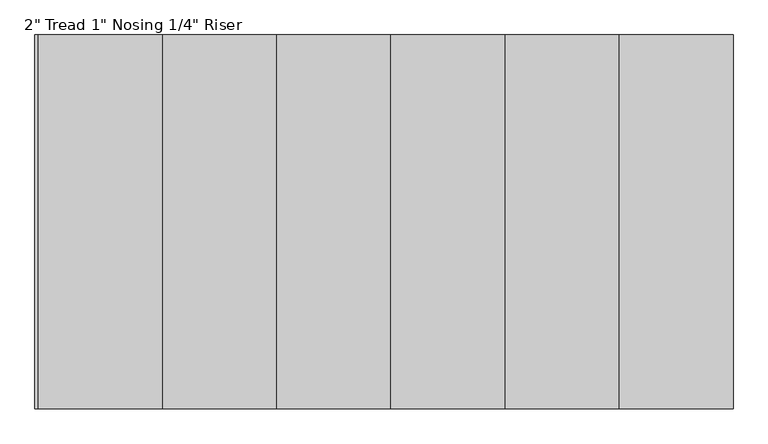
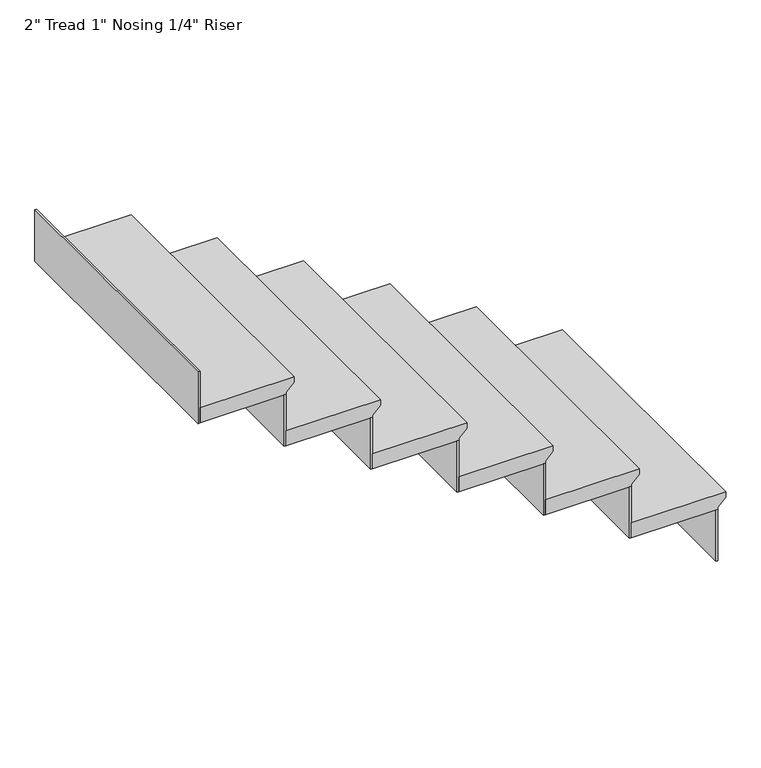
"""IFC4 building model written with IfcOpenShell, lengths in millimetres: stair flight geometry."""

from ifc_helpers import new_model, si_unit, frame, origin, place, context, project, spatial, polyline, outline, extrude, source, transform, mapped, element, save


def stair_flight_8de20f2d(model_context):
    return source(origin(), model_context, "Body", "SweptSolid", [
        extrude(outline(polyline([(5646.8210526, 8676.6463344), (5646.8210526, 8371.8463344), (5596.0210526, 8371.8463344), (5596.0210526, 8651.2463344), (5602.3710526, 8651.2463344), (5627.7710526, 8676.6463344), (5646.8210526, 8676.6463344)])), frame((0.0, -8089.9746824, 0.0), z_axis=(0.0, 1.0, 0.0), x_axis=(0.0, 0.0, 1.0)), (0.0, 0.0, 1.0), 914.4),
        extrude(outline(polyline([(8644.8963344, -7175.5746824), (8651.2463344, -7175.5746824), (8651.2463344, -8089.9746824), (8644.8963344, -8089.9746824), (8644.8963344, -7175.5746824)])), frame((0.0, 0.0, 5419.5578947), z_axis=(0.0, 0.0, 1.0), x_axis=(1.0, 0.0, 0.0)), (0.0, 0.0, 1.0), 176.4631579),
        extrude(outline(polyline([(8365.4963344, -7175.5746824), (8371.8463344, -7175.5746824), (8371.8463344, -8089.9746824), (8365.4963344, -8089.9746824), (8365.4963344, -7175.5746824)])), frame((0.0, 0.0, 5596.0210526), z_axis=(0.0, 0.0, 1.0), x_axis=(1.0, 0.0, 0.0)), (0.0, 0.0, 1.0), 176.4631579),
        extrude(outline(polyline([(5823.2842105, 8397.2463344), (5823.2842105, 8092.4463344), (5772.4842105, 8092.4463344), (5772.4842105, 8371.8463344), (5778.8342105, 8371.8463344), (5804.2342105, 8397.2463344), (5823.2842105, 8397.2463344)])), frame((0.0, -8089.9746824, 0.0), z_axis=(0.0, 1.0, 0.0), x_axis=(0.0, 0.0, 1.0)), (0.0, 0.0, 1.0), 914.4),
        extrude(outline(polyline([(8086.0963344, -7175.5746824), (8092.4463344, -7175.5746824), (8092.4463344, -8089.9746824), (8086.0963344, -8089.9746824), (8086.0963344, -7175.5746824)])), frame((0.0, 0.0, 5772.4842105), z_axis=(0.0, 0.0, 1.0), x_axis=(1.0, 0.0, 0.0)), (0.0, 0.0, 1.0), 176.4631579),
        extrude(outline(polyline([(5999.7473684, 8117.8463344), (5999.7473684, 7813.0463344), (5948.9473684, 7813.0463344), (5948.9473684, 8092.4463344), (5955.2973684, 8092.4463344), (5980.6973684, 8117.8463344), (5999.7473684, 8117.8463344)])), frame((0.0, -8089.9746824, 0.0), z_axis=(0.0, 1.0, 0.0), x_axis=(0.0, 0.0, 1.0)), (0.0, 0.0, 1.0), 914.4),
        extrude(outline(polyline([(7806.6963344, -7175.5746824), (7813.0463344, -7175.5746824), (7813.0463344, -8089.9746824), (7806.6963344, -8089.9746824), (7806.6963344, -7175.5746824)])), frame((0.0, 0.0, 5948.9473684), z_axis=(0.0, 0.0, 1.0), x_axis=(1.0, 0.0, 0.0)), (0.0, 0.0, 1.0), 176.4631579),
        extrude(outline(polyline([(6176.2105263, 7838.4463344), (6176.2105263, 7533.6463344), (6125.4105263, 7533.6463344), (6125.4105263, 7813.0463344), (6131.7605263, 7813.0463344), (6157.1605263, 7838.4463344), (6176.2105263, 7838.4463344)])), frame((0.0, -8089.9746824, 0.0), z_axis=(0.0, 1.0, 0.0), x_axis=(0.0, 0.0, 1.0)), (0.0, 0.0, 1.0), 914.4),
        extrude(outline(polyline([(7527.2963344, -7175.5746824), (7533.6463344, -7175.5746824), (7533.6463344, -8089.9746824), (7527.2963344, -8089.9746824), (7527.2963344, -7175.5746824)])), frame((0.0, 0.0, 6125.4105263), z_axis=(0.0, 0.0, 1.0), x_axis=(1.0, 0.0, 0.0)), (0.0, 0.0, 1.0), 176.4631579),
        extrude(outline(polyline([(6352.6736842, 7559.0463344), (6352.6736842, 7254.2463344), (6301.8736842, 7254.2463344), (6301.8736842, 7533.6463344), (6308.2236842, 7533.6463344), (6333.6236842, 7559.0463344), (6352.6736842, 7559.0463344)])), frame((0.0, -8089.9746824, 0.0), z_axis=(0.0, 1.0, 0.0), x_axis=(0.0, 0.0, 1.0)), (0.0, 0.0, 1.0), 914.4),
        extrude(outline(polyline([(7247.8963344, -7175.5746824), (7254.2463344, -7175.5746824), (7254.2463344, -8089.9746824), (7247.8963344, -8089.9746824), (7247.8963344, -7175.5746824)])), frame((0.0, 0.0, 6301.8736842), z_axis=(0.0, 0.0, 1.0), x_axis=(1.0, 0.0, 0.0)), (0.0, 0.0, 1.0), 176.4631579),
        extrude(outline(polyline([(6968.4963344, -7175.5746824), (6974.8463344, -7175.5746824), (6974.8463344, -8089.9746824), (6968.4963344, -8089.9746824), (6968.4963344, -7175.5746824)])), frame((0.0, 0.0, 6478.3368421), z_axis=(0.0, 0.0, 1.0), x_axis=(1.0, 0.0, 0.0)), (0.0, 0.0, 1.0), 176.4631579),
        extrude(outline(polyline([(6529.1368421, 7279.6463344), (6529.1368421, 6974.8463344), (6478.3368421, 6974.8463344), (6478.3368421, 7254.2463344), (6484.6868421, 7254.2463344), (6510.0868421, 7279.6463344), (6529.1368421, 7279.6463344)])), frame((0.0, -8089.9746824, 0.0), z_axis=(0.0, 1.0, 0.0), x_axis=(0.0, 0.0, 1.0)), (0.0, 0.0, 1.0), 914.4),
    ])


if __name__ == "__main__":
    model = new_model("IFC4")
    model_context = context("Model", 3, world=origin())
    ifc_project = project(units=[si_unit("LENGTHUNIT", "METRE", prefix="MILLI")], contexts=[model_context])
    site = spatial("IfcSite", under=ifc_project)
    building = spatial("IfcBuilding", under=site)
    placement = place(None, origin())
    stair_flight_shape = stair_flight_8de20f2d(model_context)
    element("IfcStairFlight", 1, ObjectType="2\" Tread 1\" Nosing 1/4\" Riser", at=placement, inside=building, context=model_context, shape_type="MappedRepresentation", body=[
        mapped(stair_flight_shape, transform((0.0, 0.0, 0.0), x_axis=(1.0, 0.0, 0.0), y_axis=(0.0, 1.0, 0.0), z_axis=(0.0, 0.0, 1.0))),
    ])
    save(model, "model.ifc")

# Revit data of these elements
# Element 1 (IfcStairFlight, "2\" Tread 1\" Nosing 1/4\" Riser")
#   Materials on its faces: "MARBLE STAIRS 6\""
# Materials
#   "MARBLE STAIRS 6\"": class "Generic", colour RGB 120 120 120, transparency 0, Cost = 0
